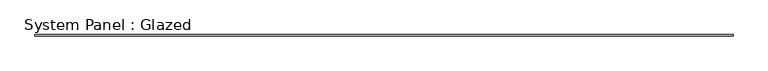
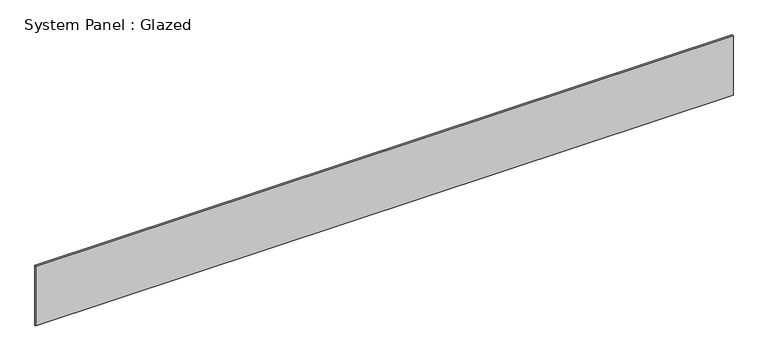
"""IFC4 building model written with IfcOpenShell, lengths in millimetres: plate geometry, System Panel : Glazed."""

from ifc_helpers import new_model, si_unit, origin, origin_with_axes, place, context, project, spatial, polyline, outline, extrude, source, transform, mapped, element, save


def system_panel_glazed_febc6b86(model_context):
    return source(origin(), model_context, "Body", "SweptSolid", [
        extrude(outline(polyline([(6379.3776373, 19.05), (-6379.3776373, 19.05), (-6379.3776373, 44.45), (6379.3776373, 44.45), (6379.3776373, 19.05)])), origin_with_axes(), (0.0, 0.0, 1.0), 1155.7),
    ])


if __name__ == "__main__":
    model = new_model("IFC4")
    model_context = context("Model", 3, world=origin())
    ifc_project = project(units=[si_unit("LENGTHUNIT", "METRE", prefix="MILLI")], contexts=[model_context])
    site = spatial("IfcSite", under=ifc_project)
    building = spatial("IfcBuilding", under=site)
    placement = place(None, origin())
    system_panel_glazed_shape = system_panel_glazed_febc6b86(model_context)
    element("IfcPlate", 1, ObjectType="System Panel : Glazed", at=placement, inside=building, context=model_context, shape_type="MappedRepresentation", body=[
        mapped(system_panel_glazed_shape, transform((0.0, 0.0, 0.0), x_axis=(1.0, 0.0, 0.0), y_axis=(0.0, 1.0, 0.0), z_axis=(0.0, 0.0, 1.0))),
    ])
    save(model, "model.ifc")

# Revit data of these elements
# Type "System Panel : Glazed"
#   Construction Type Id = "GSP4R"
#   Analytic Construction = "1/8 in Pilkington single glazing"
#   Visual Light Transmittance = 0.9
#   Solar Heat Gain Coefficient = 0.86
#   Heat Transfer Coefficient (U) = 1.18115 BTU/(h·ft²·°F)
# Element 1 (IfcPlate, "System Panel : Glazed")
#   Materials on its faces: "Glass"
# Materials
#   "Glass": class "Glass", colour RGB 0 128 192, transparency 0.75, Description = "Soda Lime Glass", Cost = 0
